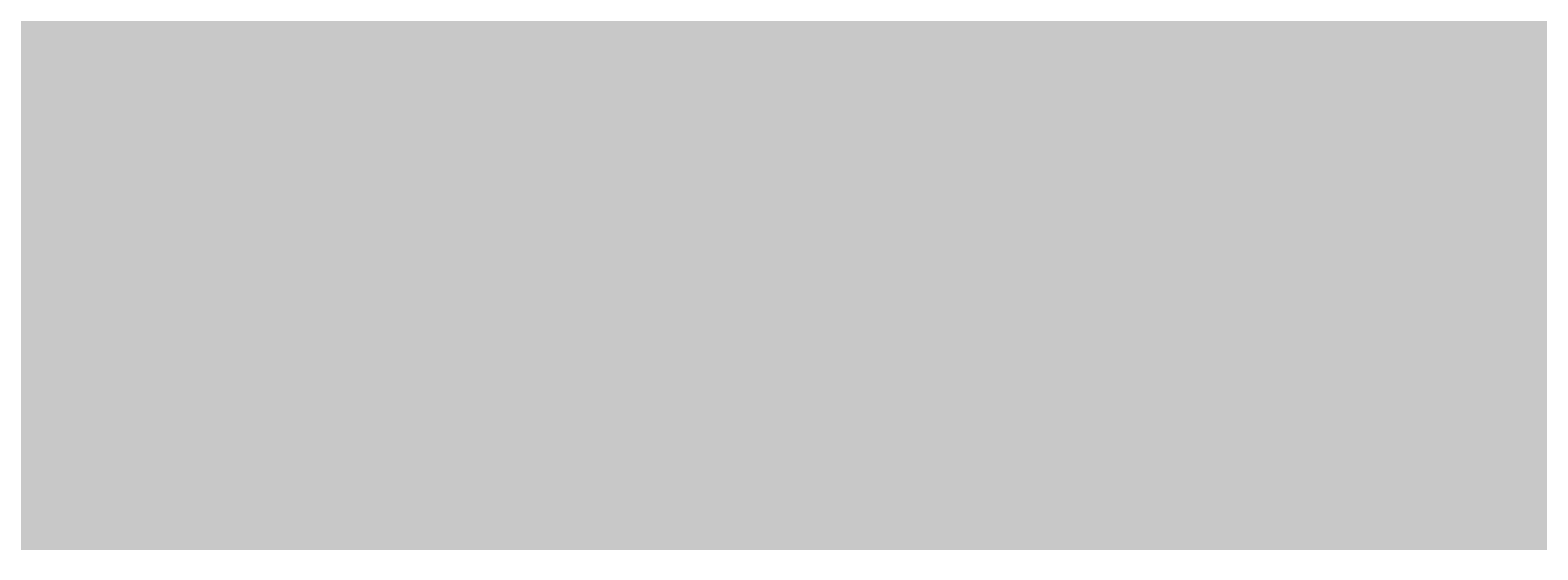
# Model space of a CAD drawing. Units: inches. Extents: x 84 to 1044, y -280 to 906.
# Tile 82 of 105: x 831 to 856, y 400 to 409. Entities that reach past the tile are written whole.
import ezdxf

# ---------------------------------------------------------------- set-up
doc = ezdxf.new("R2010")
doc.units = ezdxf.units.IN
doc.layers.add('A-ANNO-DIMS', color=2, linetype='Continuous', lineweight=18)
doc.layers.add('L-PLNT-PATT', color=9, linetype='Continuous', lineweight=9, true_color=0xafd9aa)
doc.styles.get("Standard").update_dxf_attribs({"font": 'arial.ttf'})
doc.dimstyles.get("Standard").update_dxf_attribs({"dimtxt": 0.18, "dimasz": 0.18, "dimexe": 0.18, "dimexo": 0.0625, "dimgap": 0.09, "dimtad": 0, "dimtih": 1, "dimtoh": 1, "dimdec": 4, "dimzin": 0, "dimdsep": 46, "dimtxsty": 'Standard', "dimcen": 0.09, "dimadec": 0, "dimazin": 0, "dimtfac": 1, "dimtdec": 4, "dimtofl": 0, "dimtmove": 0, "dimatfit": 3, "dimfxl": 1, "dimtolj": 1, "dimtzin": 0, "dimarcsym": 0})

# ---------------------------------------------------------------- blocks, each defined once
blk = doc.blocks.new('*D62')
at = {"layer": 'A-ANNO-DIMS', "color": 0, "lineweight": -2, "transparency": 16777216}
for p, q in [((203.179, 709.183), (203.179, 905.9)), ((896.074, 400.183), (896.074, 905.9)), ((203.359, 905.72), (549.232, 905.72)), ((895.894, 905.72), (550.021, 905.72))]:
    blk.add_line(p, q, dxfattribs=at)
at = {"layer": 'A-ANNO-DIMS', "color": 0, "transparency": 16777216}
for points in [[(203.359, 905.75), (203.359, 905.69), (203.179, 905.72)], [(895.894, 905.75), (895.894, 905.69), (896.074, 905.72)]]:
    blk.add_solid(points, dxfattribs=at)
at = {"layer": 'Defpoints', "color": 0, "transparency": 16777216}
for p in [(896.074, 905.72), (203.179, 709.12), (896.074, 400.12)]:
    blk.add_point(p, dxfattribs=at)
at = {"layer": 'A-ANNO-DIMS', "color": 0, "transparency": 16777216, "insert": (549.627, 905.72), "char_height": 0.18, "attachment_point": 5}
blk.add_mtext('\\A1;692.9', dxfattribs=at)
blk = doc.blocks.new('*D63')
at = {"layer": 'A-ANNO-DIMS', "color": 0, "lineweight": -2, "transparency": 16777216}
for p, q in [((833.136, 709.12), (1043.768, 709.12)), ((1043.588, 708.94), (1043.588, 400.302)), ((1043.588, 91.3), (1043.588, 399.938)), ((896.136, 91.12), (1043.768, 91.12))]:
    blk.add_line(p, q, dxfattribs=at)
at = {"layer": 'A-ANNO-DIMS', "color": 0, "transparency": 16777216}
for points in [[(1043.558, 708.94), (1043.618, 708.94), (1043.588, 709.12)], [(1043.558, 91.3), (1043.618, 91.3), (1043.588, 91.12)]]:
    blk.add_solid(points, dxfattribs=at)
at = {"layer": 'Defpoints', "color": 0, "transparency": 16777216}
for p in [(833.074, 709.12), (1043.588, 709.12), (896.074, 91.12)]:
    blk.add_point(p, dxfattribs=at)
at = {"layer": 'A-ANNO-DIMS', "color": 0, "transparency": 16777216, "insert": (1043.588, 400.12), "char_height": 0.18, "attachment_point": 5}
blk.add_mtext('\\A1;618', dxfattribs=at)

msp = doc.modelspace()

# ---------------------------------------------------------------- hatches: boundary and pattern name
at = {"layer": 'L-PLNT-PATT', "transparency": 33554597}
h = msp.add_hatch(color=256, dxfattribs=at)
h.dxf.hatch_style = 1
h.paths.add_polyline_path([(896.074, 511.12), (704.074, 511.12), (704.074, 491.62), (704.074, 419.62), (704.074, 400.12), (833.074, 400.12), (896.074, 400.12)])

# ---------------------------------------------------------------- dimensions: what is measured, and where the dimension line sits
at = {"layer": 'A-ANNO-DIMS'}
dim = msp.add_linear_dim(base=(896.074, 905.72), p1=(203.179, 709.12), p2=(896.074, 400.12), dimstyle='Standard', override={"dimdec": 1, "dimlfac": 1, "dimrnd": 0, "dimzin": 0, "dimdsep": 46, "dimlunit": 2}, dxfattribs=at)
dim.commit()
dim.dimension.update_dxf_attribs({"geometry": '*D62', "text_midpoint": (549.627, 905.72)})
dim = msp.add_linear_dim(base=(1043.588, 709.12), p1=(896.074, 91.12), p2=(833.074, 709.12), angle=90, dimstyle='Standard', override={"dimdec": 0, "dimlfac": 1, "dimrnd": 0, "dimzin": 0, "dimdsep": 46, "dimlunit": 2}, dxfattribs=at)
dim.commit()
dim.dimension.update_dxf_attribs({"geometry": '*D63', "text_midpoint": (1043.588, 400.12)})

doc.saveas('drawing.dxf')
